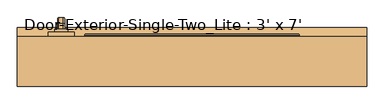
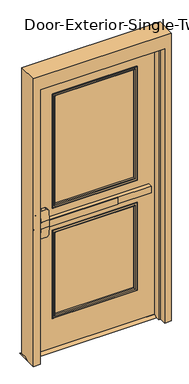
"""IFC4 building model written with IfcOpenShell, lengths in millimetres: door geometry, Door-Exterior-Single-Two_Lite : 3' x 7'."""

from ifc_helpers import new_model, si_unit, point, frame, frame_2d, origin, place, context, project, spatial, polyline, circle_curve, ellipse_curve, trimmed, segment, composite_curve, outline, extrude, faceted_brep, source, transform, mapped, element, save
from ifc_brep_helpers import plane_surface, cylinder_surface, revolved_surface, advanced_brep


def door_exterior_single_two_lite_3_x_7_37050820(model_context):
    return source(origin(), model_context, "Body", "SolidModel", [
        extrude(outline(polyline([(12.7, 12.7), (57.15, 12.7), (82.55, 0.0), (-12.7, 0.0), (12.7, 12.7)])), frame((-508.0, 0.0, 0.0), z_axis=(1.0, 0.0, 0.0), x_axis=(0.0, 1.0, 0.0)), (0.0, 0.0, 1.0), 1016.0),
        extrude(outline(polyline([(150.2833333, -25.4), (-349.25, -25.4), (-349.25, -19.05), (150.2833333, -19.05), (150.2833333, -25.4)])), frame((0.0, 0.0, 990.6), z_axis=(0.0, 0.0, 1.0), x_axis=(1.0, 0.0, 0.0)), (0.0, 0.0, 1.0), 50.8),
        advanced_brep(
        [(-412.75, -19.05, 1041.4), (-412.75, -19.05, 990.6), (-349.25, -19.05, 990.6), (400.05, -19.05, 990.6), (400.05, -19.05, 1041.4), (-349.25, -19.05, 1041.4), (400.05, 12.7, 1041.4), (400.05, 12.7, 990.6), (-349.25, 12.7, 990.6), (-349.25, 12.7, 927.1), (-368.3, 12.7, 908.05), (-393.7, 12.7, 908.05), (-412.75, 12.7, 927.1), (-412.75, 12.7, 1104.9), (-393.7, 12.7, 1123.95), (-368.3, 12.7, 1123.95), (-349.25, 12.7, 1104.9), (-349.25, 12.7, 1041.4), (-349.25, -15.8747533, 1041.4), (-412.75, -15.8747533, 1041.4), (-412.75, -10.8645731, 1104.9), (-412.75, -10.8645731, 927.1), (-412.75, -15.8747533, 990.6), (-349.25, -15.8747533, 990.6), (-349.25, -10.8645731, 927.1), (-349.25, -10.8645731, 1104.9), (-393.7, -9.361519, 1123.95), (-368.3, -9.361519, 1123.95), (-368.3, -9.361519, 908.05), (-393.7, -9.361519, 908.05)],
        [
            (0, 1),
            (1, 2),
            (2, 3),
            (3, 4),
            (4, 5),
            (5, 0),
            (6, 7),
            (7, 8),
            (8, 9),
            (9, 10, circle_curve(frame((-368.3, 12.7, 927.1), z_axis=(0.0, 1.0, 0.0), x_axis=(1.0, 0.0, 0.0)), 19.05)),
            (10, 11),
            (11, 12, circle_curve(frame((-393.7, 12.7, 927.1), z_axis=(0.0, 1.0, 0.0), x_axis=(1.0, 0.0, 0.0)), 19.05)),
            (12, 13),
            (13, 14, circle_curve(frame((-393.7, 12.7, 1104.9), z_axis=(0.0, 1.0, 0.0), x_axis=(1.0, 0.0, 0.0)), 19.05)),
            (14, 15),
            (15, 16, circle_curve(frame((-368.3, 12.7, 1104.9), z_axis=(0.0, 1.0, 0.0), x_axis=(1.0, 0.0, 0.0)), 19.05)),
            (16, 17),
            (17, 6),
            (4, 6),
            (17, 18),
            (18, 19),
            (19, 0),
            (19, 20),
            (20, 13),
            (12, 21),
            (21, 22),
            (22, 1),
            (7, 3),
            (22, 23),
            (23, 8),
            (23, 24),
            (24, 9),
            (16, 25),
            (25, 18),
            (14, 26),
            (26, 27),
            (27, 15),
            (10, 28),
            (28, 29),
            (29, 11),
            (24, 28, ellipse_curve(frame((-368.3, -10.8645731, 927.1), z_axis=(0.0, 0.9969018152893365, 0.07865602756830282), x_axis=(0.0, -0.07865602756830208, 0.9969018152893365)), 19.1092038, 19.05)),
            (27, 25, ellipse_curve(frame((-368.3, -10.8645731, 1104.9), z_axis=(0.0, 0.9969018152893376, -0.07865602756828934), x_axis=(0.0, -0.078656027568288, -0.9969018152893377)), 19.1092038, 19.05)),
            (20, 26, ellipse_curve(frame((-393.7, -10.8645731, 1104.9), z_axis=(0.0, 0.9969018152893376, -0.07865602756828934), x_axis=(0.0, -0.078656027568288, -0.9969018152893377)), 19.1092038, 19.05)),
            (29, 21, ellipse_curve(frame((-393.7, -10.8645731, 927.1), z_axis=(0.0, 0.9969018152893365, 0.07865602756830282), x_axis=(0.0, -0.07865602756830208, 0.9969018152893365)), 19.1092038, 19.05)),
        ],
        [
            plane_surface(frame((-412.75, -19.05, 1041.4), z_axis=(0.0, -1.0, 0.0), x_axis=(-1.0, 0.0, 0.0))),
            plane_surface(frame((-412.75, 12.7, 1041.4), z_axis=(0.0, 1.0, 0.0), x_axis=(1.0, 0.0, 0.0))),
            plane_surface(frame((400.05, -19.05, 1041.4), z_axis=(0.0, 0.0, 1.0), x_axis=(0.0, 1.0, 0.0))),
            plane_surface(frame((-412.75, -19.05, 1041.4), z_axis=(-1.0, 0.0, 0.0), x_axis=(0.0, 1.0, 0.0))),
            plane_surface(frame((-412.75, -19.05, 990.6), z_axis=(0.0, 0.0, -1.0), x_axis=(0.0, 1.0, 0.0))),
            plane_surface(frame((400.05, -19.05, 990.6), z_axis=(1.0, 0.0, 0.0), x_axis=(0.0, 1.0, 0.0))),
            plane_surface(frame((-349.25, -15.8747533, 927.1), z_axis=(1.0, 0.0, 0.0), x_axis=(0.0, 1.0, 0.0))),
            plane_surface(frame((-368.3, -15.8747533, 1123.95), z_axis=(0.0, 0.0, 1.0), x_axis=(0.0, 1.0, 0.0))),
            plane_surface(frame((-393.7, -15.8747533, 908.05), z_axis=(0.0, 0.0, -1.0), x_axis=(0.0, 1.0, 0.0))),
            cylinder_surface(frame((-368.3, 12.7, 927.1), z_axis=(0.0, -1.0, 0.0), x_axis=(1.0, 0.0, 0.0)), 19.05),
            cylinder_surface(frame((-368.3, 12.7, 1104.9), z_axis=(0.0, -1.0, 0.0), x_axis=(1.0, 0.0, 0.0)), 19.05),
            cylinder_surface(frame((-393.7, 12.7, 1104.9), z_axis=(0.0, -1.0, 0.0), x_axis=(1.0, 0.0, 0.0)), 19.05),
            cylinder_surface(frame((-393.7, 12.7, 927.1), z_axis=(0.0, -1.0, 0.0), x_axis=(1.0, 0.0, 0.0)), 19.05),
            plane_surface(frame((-349.25, -15.8747533, 1041.4), z_axis=(0.0, -0.9969018152893376, 0.07865602756828934), x_axis=(-1.0, 0.0, 0.0))),
            plane_surface(frame((-349.25, -9.361519, 908.05), z_axis=(0.0, -0.9969018152893365, -0.07865602756830282), x_axis=(-1.0, 0.0, 0.0))),
        ],
        [
            (0, [[1, 2, 3, 4, 5, 6]]),
            (1, [[7, 8, 9, 10, 11, 12, 13, 14, 15, 16, 17, 18]]),
            (2, [[19, -18, 20, 21, 22, -6, -5]]),
            (3, [[-1, -22, 23, 24, -13, 25, 26, 27]]),
            (4, [[28, -3, -2, -27, 29, 30, -8]]),
            (5, [[-4, -28, -7, -19]]),
            (6, [[-9, -30, 31, 32]]),
            (6, [[-17, 33, 34, -20]]),
            (7, [[-15, 35, 36, 37]]),
            (8, [[-11, 38, 39, 40]]),
            (9, [[-10, -32, 41, -38]]),
            (10, [[-16, -37, 42, -33]]),
            (11, [[-14, -24, 43, -35]]),
            (12, [[-12, -40, 44, -25]]),
            (13, [[-21, -34, -42, -36, -43, -23]]),
            (14, [[-26, -44, -39, -41, -31, -29]]),
        ],
    ),
        advanced_brep(
        [(-391.0, 69.85, 1017.190625), (-391.0, 69.85, 1014.809375), (-387.428125, 69.85, 1011.2375), (-374.5715406, 69.85, 1011.2375), (-371.0, 69.85, 1014.8090406), (-371.0, 69.85, 1017.190625), (-374.571875, 69.85, 1020.7625), (-387.428125, 69.85, 1020.7625), (-391.0, 69.85, 887.809375), (-387.428125, 69.85, 884.2375), (-374.571875, 69.85, 884.2375), (-371.0, 69.85, 887.809375), (-371.0, 69.85, 890.1909594), (-374.5715406, 69.85, 893.7625), (-387.428125, 69.85, 893.7625), (-391.0, 69.85, 890.190625), (-391.0, 95.25, 1017.190625), (-391.0, 109.140625, 1003.3), (-391.0, 109.140625, 901.7), (-391.0, 95.25, 887.809375), (-391.0, 95.25, 890.190625), (-391.0, 106.759375, 901.7), (-391.0, 106.759375, 1003.3), (-391.0, 95.25, 1014.809375), (-387.428125, 95.25, 1011.2375), (-374.5715406, 95.25, 1011.2375), (-371.0, 95.25, 1014.8090406), (-371.0, 106.7590406, 1003.3), (-371.0, 106.7590406, 901.7), (-371.0, 95.25, 890.1909594), (-371.0, 95.25, 887.809375), (-371.0, 109.140625, 901.7), (-371.0, 109.140625, 1003.3), (-371.0, 95.25, 1017.190625), (-374.571875, 95.25, 1020.7625), (-387.428125, 95.25, 1020.7625), (-387.428125, 103.1875, 1003.3), (-374.5715406, 103.1875, 1003.3), (-374.571875, 112.7125, 1003.3), (-387.428125, 112.7125, 1003.3), (-387.428125, 103.1875, 901.7), (-374.5715406, 103.1875, 901.7), (-374.571875, 112.7125, 901.7), (-387.428125, 112.7125, 901.7), (-387.428125, 95.25, 893.7625), (-374.5715406, 95.25, 893.7625), (-374.571875, 95.25, 884.2375), (-387.428125, 95.25, 884.2375)],
        [
            (0, 1),
            (1, 2, circle_curve(frame((-387.428125, 69.85, 1014.809375), z_axis=(0.0, -1.0, 0.0), x_axis=(0.0, 0.0, 1.0)), 3.571875)),
            (2, 3),
            (3, 4, circle_curve(frame((-374.5715406, 69.85, 1014.8090406), z_axis=(0.0, -1.0, 0.0), x_axis=(0.0, 0.0, 1.0)), 3.5715406)),
            (4, 5),
            (5, 6, circle_curve(frame((-374.571875, 69.85, 1017.190625), z_axis=(0.0, -1.0, 0.0), x_axis=(0.0, 0.0, 1.0)), 3.571875)),
            (6, 7),
            (7, 0, circle_curve(frame((-387.428125, 69.85, 1017.190625), z_axis=(0.0, -1.0, 0.0), x_axis=(0.0, 0.0, 1.0)), 3.571875)),
            (8, 9, circle_curve(frame((-387.428125, 69.85, 887.809375), z_axis=(0.0, -1.0, 0.0), x_axis=(0.0, 0.0, -1.0)), 3.571875)),
            (9, 10),
            (10, 11, circle_curve(frame((-374.571875, 69.85, 887.809375), z_axis=(0.0, -1.0, 0.0), x_axis=(0.0, 0.0, -1.0)), 3.571875)),
            (11, 12),
            (12, 13, circle_curve(frame((-374.5715406, 69.85, 890.1909594), z_axis=(0.0, -1.0, 0.0), x_axis=(0.0, 0.0, -1.0)), 3.5715406)),
            (13, 14),
            (14, 15, circle_curve(frame((-387.428125, 69.85, 890.190625), z_axis=(0.0, -1.0, 0.0), x_axis=(0.0, 0.0, -1.0)), 3.571875)),
            (15, 8),
            (0, 16),
            (16, 17, circle_curve(frame((-391.0, 95.25, 1003.3), z_axis=(-1.0, 0.0, 0.0), x_axis=(0.0, 0.0, 1.0)), 13.890625)),
            (17, 18),
            (18, 19, circle_curve(frame((-391.0, 95.25, 901.7), z_axis=(-1.0, 0.0, 0.0), x_axis=(0.0, 1.0, 0.0)), 13.890625)),
            (19, 8),
            (15, 20),
            (20, 21, circle_curve(frame((-391.0, 95.25, 901.7), z_axis=(1.0, 0.0, 0.0), x_axis=(0.0, 1.0, 0.0)), 11.509375)),
            (21, 22),
            (22, 23, circle_curve(frame((-391.0, 95.25, 1003.3), z_axis=(1.0, 0.0, 0.0), x_axis=(0.0, 0.0, 1.0)), 11.509375)),
            (23, 1),
            (23, 24, circle_curve(frame((-387.428125, 95.25, 1014.809375), z_axis=(0.0, -1.0, 0.0), x_axis=(0.0, 0.0, 1.0)), 3.571875)),
            (24, 2),
            (24, 25),
            (25, 3),
            (25, 26, circle_curve(frame((-374.5715406, 95.25, 1014.8090406), z_axis=(0.0, -1.0, 0.0), x_axis=(0.0, 0.0, 1.0)), 3.5715406)),
            (26, 4),
            (26, 27, circle_curve(frame((-371.0, 95.25, 1003.3), z_axis=(-1.0, 0.0, 0.0), x_axis=(0.0, 0.0, 1.0)), 11.5090406)),
            (27, 28),
            (28, 29, circle_curve(frame((-371.0, 95.25, 901.7), z_axis=(-1.0, 0.0, 0.0), x_axis=(0.0, 1.0, 0.0)), 11.5090406)),
            (29, 12),
            (11, 30),
            (30, 31, circle_curve(frame((-371.0, 95.25, 901.7), z_axis=(1.0, 0.0, 0.0), x_axis=(0.0, 1.0, 0.0)), 13.890625)),
            (31, 32),
            (32, 33, circle_curve(frame((-371.0, 95.25, 1003.3), z_axis=(1.0, 0.0, 0.0), x_axis=(0.0, 0.0, 1.0)), 13.890625)),
            (33, 5),
            (33, 34, circle_curve(frame((-374.571875, 95.25, 1017.190625), z_axis=(0.0, -1.0, 0.0), x_axis=(0.0, 0.0, 1.0)), 3.571875)),
            (34, 6),
            (34, 35),
            (35, 7),
            (35, 16, circle_curve(frame((-387.428125, 95.25, 1017.190625), z_axis=(0.0, -1.0, 0.0), x_axis=(0.0, 0.0, 1.0)), 3.571875)),
            (36, 24, circle_curve(frame((-387.428125, 95.25, 1003.3), z_axis=(1.0, 0.0, 0.0), x_axis=(0.0, 0.0, 1.0)), 7.9375)),
            (22, 36, circle_curve(frame((-387.428125, 106.759375, 1003.3), z_axis=(0.0, 0.0, 1.0), x_axis=(0.0, 1.0, 0.0)), 3.571875)),
            (37, 25, circle_curve(frame((-374.5715406, 95.25, 1003.3), z_axis=(1.0, 0.0, 0.0), x_axis=(0.0, 0.0, 1.0)), 7.9375)),
            (36, 37),
            (37, 27, circle_curve(frame((-374.5715406, 106.7590406, 1003.3), z_axis=(0.0, 0.0, 1.0), x_axis=(0.0, 1.0, 0.0)), 3.5715406)),
            (38, 34, circle_curve(frame((-374.571875, 95.25, 1003.3), z_axis=(1.0, 0.0, 0.0), x_axis=(0.0, 0.0, 1.0)), 17.4625)),
            (32, 38, circle_curve(frame((-374.571875, 109.140625, 1003.3), z_axis=(0.0, 0.0, 1.0), x_axis=(0.0, 1.0, 0.0)), 3.571875)),
            (39, 35, circle_curve(frame((-387.428125, 95.25, 1003.3), z_axis=(1.0, 0.0, 0.0), x_axis=(0.0, 0.0, 1.0)), 17.4625)),
            (38, 39),
            (39, 17, circle_curve(frame((-387.428125, 109.140625, 1003.3), z_axis=(0.0, 0.0, 1.0), x_axis=(0.0, 1.0, 0.0)), 3.571875)),
            (21, 40, circle_curve(frame((-387.428125, 106.759375, 901.7), z_axis=(0.0, 0.0, 1.0), x_axis=(0.0, 1.0, 0.0)), 3.571875)),
            (40, 36),
            (40, 41),
            (41, 37),
            (41, 28, circle_curve(frame((-374.5715406, 106.7590406, 901.7), z_axis=(0.0, 0.0, 1.0), x_axis=(0.0, 1.0, 0.0)), 3.5715406)),
            (31, 42, circle_curve(frame((-374.571875, 109.140625, 901.7), z_axis=(0.0, 0.0, 1.0), x_axis=(0.0, 1.0, 0.0)), 3.571875)),
            (42, 38),
            (42, 43),
            (43, 39),
            (43, 18, circle_curve(frame((-387.428125, 109.140625, 901.7), z_axis=(0.0, 0.0, 1.0), x_axis=(0.0, 1.0, 0.0)), 3.571875)),
            (44, 40, circle_curve(frame((-387.428125, 95.25, 901.7), z_axis=(1.0, 0.0, 0.0), x_axis=(0.0, 1.0, 0.0)), 7.9375)),
            (20, 44, circle_curve(frame((-387.428125, 95.25, 890.190625), z_axis=(0.0, 1.0, 0.0), x_axis=(0.0, 0.0, -1.0)), 3.571875)),
            (45, 41, circle_curve(frame((-374.5715406, 95.25, 901.7), z_axis=(1.0, 0.0, 0.0), x_axis=(0.0, 1.0, 0.0)), 7.9375)),
            (44, 45),
            (45, 29, circle_curve(frame((-374.5715406, 95.25, 890.1909594), z_axis=(0.0, 1.0, 0.0), x_axis=(0.0, 0.0, -1.0)), 3.5715406)),
            (46, 42, circle_curve(frame((-374.571875, 95.25, 901.7), z_axis=(1.0, 0.0, 0.0), x_axis=(0.0, 1.0, 0.0)), 17.4625)),
            (30, 46, circle_curve(frame((-374.571875, 95.25, 887.809375), z_axis=(0.0, 1.0, 0.0), x_axis=(0.0, 0.0, -1.0)), 3.571875)),
            (47, 43, circle_curve(frame((-387.428125, 95.25, 901.7), z_axis=(1.0, 0.0, 0.0), x_axis=(0.0, 1.0, 0.0)), 17.4625)),
            (46, 47),
            (47, 19, circle_curve(frame((-387.428125, 95.25, 887.809375), z_axis=(0.0, 1.0, 0.0), x_axis=(0.0, 0.0, -1.0)), 3.571875)),
            (14, 44),
            (13, 45),
            (10, 46),
            (9, 47),
        ],
        [
            plane_surface(frame((-381.0, 69.85, 1016.0), z_axis=(0.0, -1.0, 0.0), x_axis=(1.0, 0.0, 0.0))),
            plane_surface(frame((-381.0, 69.85, 889.0), z_axis=(0.0, -1.0, 0.0), x_axis=(1.0, 0.0, 0.0))),
            plane_surface(frame((-391.0, 69.85, 1017.190625), z_axis=(-1.0, 0.0, 0.0), x_axis=(0.0, 1.0, 0.0))),
            cylinder_surface(frame((-387.428125, 69.85, 1014.809375), z_axis=(0.0, -1.0, 0.0), x_axis=(0.0, 0.0, 1.0)), 3.571875),
            plane_surface(frame((-387.428125, 69.85, 1011.2375), z_axis=(0.0, 0.0, -1.0), x_axis=(0.0, 1.0, 0.0))),
            cylinder_surface(frame((-374.5715406, 69.85, 1014.8090406), z_axis=(0.0, -1.0, 0.0), x_axis=(0.0, 0.0, 1.0)), 3.5715406),
            plane_surface(frame((-371.0, 69.85, 1014.8090406), z_axis=(1.0, 0.0, 0.0), x_axis=(0.0, 1.0, 0.0))),
            cylinder_surface(frame((-374.571875, 69.85, 1017.190625), z_axis=(0.0, -1.0, 0.0), x_axis=(0.0, 0.0, 1.0)), 3.571875),
            plane_surface(frame((-374.571875, 69.85, 1020.7625), z_axis=(0.0, 0.0, 1.0), x_axis=(0.0, 1.0, 0.0))),
            cylinder_surface(frame((-387.428125, 69.85, 1017.190625), z_axis=(0.0, -1.0, 0.0), x_axis=(0.0, 0.0, 1.0)), 3.571875),
            revolved_surface(trimmed(ellipse_curve(frame((-387.428125, 95.25, 1014.809375), z_axis=(0.0, -1.0, 0.0), x_axis=(0.0, 0.0, 1.0)), 3.571875, 3.571875), [point((-391.0, 95.25, 1014.809375))], [point((-387.428125, 95.25, 1011.2375))], True, "CARTESIAN"), (-381.0, 95.25, 1003.3), (-1.0, 0.0, 0.0)),
            revolved_surface(polyline([(-387.428125, 95.25, 1011.2375), (-374.5715406, 95.25, 1011.2375)]), (-381.0, 95.25, 1003.3), (-1.0, 0.0, 0.0)),
            revolved_surface(trimmed(ellipse_curve(frame((-374.5715406, 95.25, 1014.8090406), z_axis=(0.0, -1.0, 0.0), x_axis=(0.0, 0.0, 1.0)), 3.5715406, 3.5715406), [point((-374.5715406, 95.25, 1011.2375))], [point((-371.0, 95.25, 1014.8090406))], True, "CARTESIAN"), (-381.0, 95.25, 1003.3), (-1.0, 0.0, 0.0)),
            revolved_surface(trimmed(ellipse_curve(frame((-374.571875, 95.25, 1017.190625), z_axis=(0.0, -1.0, 0.0), x_axis=(0.0, 0.0, 1.0)), 3.571875, 3.571875), [point((-371.0, 95.25, 1017.190625))], [point((-374.571875, 95.25, 1020.7625))], True, "CARTESIAN"), (-381.0, 95.25, 1003.3), (-1.0, 0.0, 0.0)),
            cylinder_surface(frame((-381.0, 95.25, 1003.3), z_axis=(-1.0, 0.0, 0.0), x_axis=(0.0, 0.0, 1.0)), 17.4625),
            revolved_surface(trimmed(ellipse_curve(frame((-387.428125, 95.25, 1017.190625), z_axis=(0.0, -1.0, 0.0), x_axis=(0.0, 0.0, 1.0)), 3.571875, 3.571875), [point((-387.428125, 95.25, 1020.7625))], [point((-391.0, 95.25, 1017.190625))], True, "CARTESIAN"), (-381.0, 95.25, 1003.3), (-1.0, 0.0, 0.0)),
            cylinder_surface(frame((-387.428125, 106.759375, 1003.3), z_axis=(0.0, 0.0, 1.0), x_axis=(0.0, 1.0, 0.0)), 3.571875),
            plane_surface(frame((-387.428125, 103.1875, 1003.3), z_axis=(0.0, -1.0, 0.0), x_axis=(0.0, 0.0, -1.0))),
            cylinder_surface(frame((-374.5715406, 106.7590406, 1003.3), z_axis=(0.0, 0.0, 1.0), x_axis=(0.0, 1.0, 0.0)), 3.5715406),
            cylinder_surface(frame((-374.571875, 109.140625, 1003.3), z_axis=(0.0, 0.0, 1.0), x_axis=(0.0, 1.0, 0.0)), 3.571875),
            plane_surface(frame((-374.571875, 112.7125, 1003.3), z_axis=(0.0, 1.0, 0.0), x_axis=(0.0, 0.0, -1.0))),
            cylinder_surface(frame((-387.428125, 109.140625, 1003.3), z_axis=(0.0, 0.0, 1.0), x_axis=(0.0, 1.0, 0.0)), 3.571875),
            revolved_surface(trimmed(ellipse_curve(frame((-387.428125, 106.759375, 901.7), z_axis=(0.0, 0.0, 1.0), x_axis=(0.0, 1.0, 0.0)), 3.571875, 3.571875), [point((-391.0, 106.759375, 901.7))], [point((-387.428125, 103.1875, 901.7))], True, "CARTESIAN"), (-381.0, 95.25, 901.7), (-1.0, 0.0, 0.0)),
            revolved_surface(polyline([(-387.428125, 103.1875, 901.7), (-374.5715406, 103.1875, 901.7)]), (-381.0, 95.25, 901.7), (-1.0, 0.0, 0.0)),
            revolved_surface(trimmed(ellipse_curve(frame((-374.5715406, 106.7590406, 901.7), z_axis=(0.0, 0.0, 1.0), x_axis=(0.0, 1.0, 0.0)), 3.5715406, 3.5715406), [point((-374.5715406, 103.1875, 901.7))], [point((-371.0, 106.7590406, 901.7))], True, "CARTESIAN"), (-381.0, 95.25, 901.7), (-1.0, 0.0, 0.0)),
            revolved_surface(trimmed(ellipse_curve(frame((-374.571875, 109.140625, 901.7), z_axis=(0.0, 0.0, 1.0), x_axis=(0.0, 1.0, 0.0)), 3.571875, 3.571875), [point((-371.0, 109.140625, 901.7))], [point((-374.571875, 112.7125, 901.7))], True, "CARTESIAN"), (-381.0, 95.25, 901.7), (-1.0, 0.0, 0.0)),
            cylinder_surface(frame((-381.0, 95.25, 901.7), z_axis=(-1.0, 0.0, 0.0), x_axis=(0.0, 1.0, 0.0)), 17.4625),
            revolved_surface(trimmed(ellipse_curve(frame((-387.428125, 109.140625, 901.7), z_axis=(0.0, 0.0, 1.0), x_axis=(0.0, 1.0, 0.0)), 3.571875, 3.571875), [point((-387.428125, 112.7125, 901.7))], [point((-391.0, 109.140625, 901.7))], True, "CARTESIAN"), (-381.0, 95.25, 901.7), (-1.0, 0.0, 0.0)),
            cylinder_surface(frame((-387.428125, 95.25, 890.190625), z_axis=(0.0, 1.0, 0.0), x_axis=(0.0, 0.0, -1.0)), 3.571875),
            plane_surface(frame((-387.428125, 95.25, 893.7625), z_axis=(0.0, 0.0, 1.0), x_axis=(0.0, -1.0, 0.0))),
            cylinder_surface(frame((-374.5715406, 95.25, 890.1909594), z_axis=(0.0, 1.0, 0.0), x_axis=(0.0, 0.0, -1.0)), 3.5715406),
            cylinder_surface(frame((-374.571875, 95.25, 887.809375), z_axis=(0.0, 1.0, 0.0), x_axis=(0.0, 0.0, -1.0)), 3.571875),
            plane_surface(frame((-374.571875, 95.25, 884.2375), z_axis=(0.0, 0.0, -1.0), x_axis=(0.0, -1.0, 0.0))),
            cylinder_surface(frame((-387.428125, 95.25, 887.809375), z_axis=(0.0, 1.0, 0.0), x_axis=(0.0, 0.0, -1.0)), 3.571875),
        ],
        [
            (0, [[1, 2, 3, 4, 5, 6, 7, 8]]),
            (1, [[9, 10, 11, 12, 13, 14, 15, 16]]),
            (2, [[-1, 17, 18, 19, 20, 21, -16, 22, 23, 24, 25, 26]]),
            (3, [[-2, -26, 27, 28]]),
            (4, [[-3, -28, 29, 30]]),
            (5, [[-4, -30, 31, 32]]),
            (6, [[-5, -32, 33, 34, 35, 36, -12, 37, 38, 39, 40, 41]]),
            (7, [[-6, -41, 42, 43]]),
            (8, [[-7, -43, 44, 45]]),
            (9, [[-8, -45, 46, -17]]),
            (10, [[47, -27, -25, 48]]),
            (11, [[49, -29, -47, 50]]),
            (12, [[-33, -31, -49, 51]]),
            (13, [[52, -42, -40, 53]]),
            (14, [[54, -44, -52, 55]]),
            (15, [[-18, -46, -54, 56]]),
            (16, [[-48, -24, 57, 58]]),
            (17, [[-50, -58, 59, 60]]),
            (18, [[-51, -60, 61, -34]]),
            (19, [[-53, -39, 62, 63]]),
            (20, [[-55, -63, 64, 65]]),
            (21, [[-56, -65, 66, -19]]),
            (22, [[67, -57, -23, 68]]),
            (23, [[69, -59, -67, 70]]),
            (24, [[-35, -61, -69, 71]]),
            (25, [[72, -62, -38, 73]]),
            (26, [[74, -64, -72, 75]]),
            (27, [[-20, -66, -74, 76]]),
            (28, [[-68, -22, -15, 77]]),
            (29, [[-70, -77, -14, 78]]),
            (30, [[-71, -78, -13, -36]]),
            (31, [[-73, -37, -11, 79]]),
            (32, [[-75, -79, -10, 80]]),
            (33, [[-76, -80, -9, -21]]),
        ],
    ),
        extrude(outline(composite_curve([segment(trimmed(circle_curve(frame_2d((1117.6, -381.0)), 19.0), [point((1117.6, -400.0))], [point((1117.6, -362.0))], False, "CARTESIAN"), True, "CONTINUOUS"), segment(trimmed(circle_curve(frame_2d((1117.6, -381.0)), 19.0), [point((1117.6, -362.0))], [point((1117.6, -400.0))], False, "CARTESIAN"), True, "CONTINUOUS")], self_intersect=False)), frame((0.0, 69.85, 0.0), z_axis=(0.0, 1.0, 0.0), x_axis=(0.0, 0.0, 1.0)), (0.0, 0.0, 1.0), 8.73125),
        extrude(outline(composite_curve([segment(trimmed(circle_curve(frame_2d((1113.0338574, -381.0)), 89.3016225), [point((1193.8, -342.9))], [point((1193.8, -419.1))], False, "CARTESIAN"), True, "CONTINUOUS"), segment(polyline([(1193.8, -419.1), (838.2, -419.1)]), True, "CONTINUOUS"), segment(trimmed(circle_curve(frame_2d((918.9661426, -381.0)), 89.3016225), [point((838.2, -419.1))], [point((838.2, -342.9))], False, "CARTESIAN"), True, "CONTINUOUS"), segment(polyline([(838.2, -342.9), (1193.8, -342.9)]), True, "CONTINUOUS")], self_intersect=False)), frame((0.0, 57.15, 0.0), z_axis=(0.0, 1.0, 0.0), x_axis=(0.0, 0.0, 1.0)), (0.0, 0.0, 1.0), 12.7),
        extrude(outline(polyline([(2133.6, -457.2), (12.7, -457.2), (12.7, 457.2), (2133.6, 457.2), (2133.6, -457.2)]), holes=[polyline([(1981.2, -304.8), (1981.2, 304.8), (1111.25, 304.8), (1111.25, -304.8), (1981.2, -304.8)]), polyline([(920.75, -304.8), (920.75, 304.8), (254.0, 304.8), (254.0, -304.8), (920.75, -304.8)])]), frame((0.0, 12.7, 0.0), z_axis=(0.0, 1.0, 0.0), x_axis=(0.0, 0.0, 1.0)), (0.0, 0.0, 1.0), 44.45),
        faceted_brep([(457.2, 7.9375, 0.0), (457.2, 57.15, 0.0), (508.0, 57.15, 0.0), (508.0, -88.9, 0.0), (457.2, -88.9, 0.0), (457.2, -39.6875, 0.0), (441.325, -39.6875, 0.0), (441.325, 7.9375, 0.0), (457.2, 7.9375, 2133.6), (457.2, 57.15, 2133.6), (-457.2, 57.15, 2133.6), (-457.2, 57.15, 0.0), (-508.0, 57.15, 0.0), (-508.0, 57.15, 2235.2), (508.0, 57.15, 2235.2), (508.0, -88.9, 2235.2), (-508.0, -88.9, 2235.2), (-508.0, -88.9, 0.0), (-457.2, -88.9, 0.0), (-457.2, -88.9, 2133.6), (457.2, -88.9, 2133.6), (457.2, -39.6875, 2133.6), (-457.2, -39.6875, 2133.6), (-457.2, -39.6875, 0.0), (-441.325, -39.6875, 0.0), (-441.325, -39.6875, 2117.725), (441.325, -39.6875, 2117.725), (441.325, 7.9375, 2117.725), (-441.325, 7.9375, 2117.725), (-441.325, 7.9375, 0.0), (-457.2, 7.9375, 0.0), (-457.2, 7.9375, 2133.6)], [[[0, 1, 2, 3, 4, 5, 6, 7]], [[1, 0, 8, 9]], [[2, 1, 9, 10, 11, 12, 13, 14]], [[3, 2, 14, 15]], [[4, 3, 15, 16, 17, 18, 19, 20]], [[5, 4, 20, 21]], [[6, 5, 21, 22, 23, 24, 25, 26]], [[7, 6, 26, 27]], [[0, 7, 27, 28, 29, 30, 31, 8]], [[9, 8, 31, 10]], [[20, 19, 22, 21]], [[26, 25, 28, 27]], [[12, 11, 30, 29, 24, 23, 18, 17]], [[11, 10, 31, 30]], [[13, 12, 17, 16]], [[19, 18, 23, 22]], [[25, 24, 29, 28]], [[15, 14, 13, 16]]]),
        extrude(outline(polyline([(304.8, 25.4), (-304.8, 25.4), (-304.8, 44.45), (304.8, 44.45), (304.8, 25.4)])), frame((0.0, 0.0, 1111.25), z_axis=(0.0, 0.0, 1.0), x_axis=(1.0, 0.0, 0.0)), (0.0, 0.0, 1.0), 869.95),
        extrude(outline(polyline([(304.8, 25.4), (-304.8, 25.4), (-304.8, 44.45), (304.8, 44.45), (304.8, 25.4)])), frame((0.0, 0.0, 254.0), z_axis=(0.0, 0.0, 1.0), x_axis=(1.0, 0.0, 0.0)), (0.0, 0.0, 1.0), 666.75),
        advanced_brep(
        [(-304.8, 44.45, 1981.2), (-304.8, 57.15, 1981.2), (-304.8, 57.15, 1111.25), (-304.8, 44.45, 1111.25), (-292.8, 58.15, 1969.2), (-292.8, 44.45, 1969.2), (-292.8, 44.45, 1123.25), (-292.8, 58.15, 1123.25), (-297.8, 63.15, 1974.2), (-297.8, 63.15, 1118.25), (-312.8, 61.15, 1989.2), (-310.8, 63.15, 1987.2), (-310.8, 63.15, 1105.25), (-312.8, 61.15, 1103.25), (-312.8, 57.15, 1989.2), (-312.8, 57.15, 1103.25), (304.8, 57.15, 1111.25), (304.8, 44.45, 1111.25), (292.8, 44.45, 1123.25), (292.8, 58.15, 1123.25), (297.8, 63.15, 1118.25), (310.8, 63.15, 1105.25), (312.8, 61.15, 1103.25), (312.8, 57.15, 1103.25), (304.8, 57.15, 1981.2), (304.8, 44.45, 1981.2), (292.8, 44.45, 1969.2), (292.8, 58.15, 1969.2), (297.8, 63.15, 1974.2), (310.8, 63.15, 1987.2), (312.8, 61.15, 1989.2), (312.8, 57.15, 1989.2)],
        [
            (0, 1),
            (1, 2),
            (2, 3),
            (3, 0),
            (4, 5),
            (5, 6),
            (6, 7),
            (7, 4),
            (8, 4, ellipse_curve(frame((-297.8, 58.15, 1974.2), z_axis=(-0.7071067811865475, 0.0, -0.7071067811865475), x_axis=(-0.7071067811865474, 0.0, 0.7071067811865476)), 7.0710678, 5.0)),
            (7, 9, ellipse_curve(frame((-297.8, 58.15, 1118.25), z_axis=(-0.7071067811865475, 0.0, 0.7071067811865475), x_axis=(0.7071067811865474, 0.0, 0.7071067811865476)), 7.0710678, 5.0)),
            (9, 8),
            (10, 11, ellipse_curve(frame((-310.8, 61.15, 1987.2), z_axis=(-0.7071067811865475, 0.0, -0.7071067811865475), x_axis=(-0.7071067811865474, 0.0, 0.7071067811865476)), 2.8284271, 2.0)),
            (11, 12),
            (12, 13, ellipse_curve(frame((-310.8, 61.15, 1105.25), z_axis=(-0.7071067811865475, 0.0, 0.7071067811865475), x_axis=(0.7071067811865474, 0.0, 0.7071067811865476)), 2.8284271, 2.0)),
            (13, 10),
            (14, 10),
            (13, 15),
            (15, 14),
            (2, 16),
            (16, 17),
            (17, 3),
            (6, 18),
            (18, 19),
            (19, 7),
            (19, 20, ellipse_curve(frame((297.8, 58.15, 1118.25), z_axis=(-0.7071067811865475, 0.0, -0.7071067811865475), x_axis=(-0.7071067811865476, 0.0, 0.7071067811865474)), 7.0710678, 5.0)),
            (20, 9),
            (12, 21),
            (21, 22, ellipse_curve(frame((310.8, 61.15, 1105.25), z_axis=(-0.7071067811865475, 0.0, -0.7071067811865475), x_axis=(-0.7071067811865476, 0.0, 0.7071067811865474)), 2.8284271, 2.0)),
            (22, 13),
            (22, 23),
            (23, 15),
            (16, 24),
            (24, 25),
            (25, 17),
            (18, 26),
            (26, 27),
            (27, 19),
            (27, 28, ellipse_curve(frame((297.8, 58.15, 1974.2), z_axis=(0.7071067811865475, 0.0, -0.7071067811865475), x_axis=(-0.7071067811865474, 0.0, -0.7071067811865476)), 7.0710678, 5.0)),
            (28, 20),
            (21, 29),
            (29, 30, ellipse_curve(frame((310.8, 61.15, 1987.2), z_axis=(0.7071067811865475, 0.0, -0.7071067811865475), x_axis=(-0.7071067811865474, 0.0, -0.7071067811865476)), 2.8284271, 2.0)),
            (30, 22),
            (30, 31),
            (31, 23),
            (31, 14),
            (1, 24),
            (0, 25),
            (5, 26),
            (4, 27),
            (8, 28),
            (11, 29),
            (10, 30),
        ],
        [
            plane_surface(frame((-304.8, 57.15, 1981.2), z_axis=(-1.0, 0.0, 0.0), x_axis=(0.0, 0.0, -1.0))),
            plane_surface(frame((-292.8, 44.45, 1969.2), z_axis=(1.0, 0.0, 0.0), x_axis=(0.0, 0.0, -1.0))),
            cylinder_surface(frame((-297.8, 58.15, 1981.2), z_axis=(0.0, 0.0, 1.0), x_axis=(-1.0, 0.0, 0.0)), 5.0),
            cylinder_surface(frame((-310.8, 61.15, 1981.2), z_axis=(0.0, 0.0, 1.0), x_axis=(-1.0, 0.0, 0.0)), 2.0),
            plane_surface(frame((-312.8, 61.15, 1989.2), z_axis=(-1.0, 0.0, 0.0), x_axis=(0.0, 0.0, -1.0))),
            plane_surface(frame((-304.8, 57.15, 1111.25), z_axis=(0.0, 0.0, -1.0), x_axis=(1.0, 0.0, 0.0))),
            plane_surface(frame((-292.8, 44.45, 1123.25), z_axis=(0.0, 0.0, 1.0), x_axis=(1.0, 0.0, 0.0))),
            cylinder_surface(frame((-304.8, 58.15, 1118.25), z_axis=(-1.0, 0.0, 0.0), x_axis=(0.0, 0.0, -1.0)), 5.0),
            cylinder_surface(frame((-304.8, 61.15, 1105.25), z_axis=(-1.0, 0.0, 0.0), x_axis=(0.0, 0.0, -1.0)), 2.0),
            plane_surface(frame((-312.8, 61.15, 1103.25), z_axis=(0.0, 0.0, -1.0), x_axis=(1.0, 0.0, 0.0))),
            plane_surface(frame((304.8, 57.15, 1111.25), z_axis=(1.0, 0.0, 0.0), x_axis=(0.0, 0.0, 1.0))),
            plane_surface(frame((292.8, 44.45, 1123.25), z_axis=(-1.0, 0.0, 0.0), x_axis=(0.0, 0.0, 1.0))),
            cylinder_surface(frame((297.8, 58.15, 1111.25), z_axis=(0.0, 0.0, -1.0), x_axis=(1.0, 0.0, 0.0)), 5.0),
            cylinder_surface(frame((310.8, 61.15, 1111.25), z_axis=(0.0, 0.0, -1.0), x_axis=(1.0, 0.0, 0.0)), 2.0),
            plane_surface(frame((312.8, 61.15, 1103.25), z_axis=(1.0, 0.0, 0.0), x_axis=(0.0, 0.0, 1.0))),
            plane_surface(frame((312.8, 57.15, 1989.2), z_axis=(0.0, -1.0, 0.0), x_axis=(-1.0, 0.0, 0.0))),
            plane_surface(frame((304.8, 57.15, 1981.2), z_axis=(0.0, 0.0, 1.0), x_axis=(-1.0, 0.0, 0.0))),
            plane_surface(frame((304.8, 44.45, 1981.2), z_axis=(0.0, -1.0, 0.0), x_axis=(-1.0, 0.0, 0.0))),
            plane_surface(frame((292.8, 44.45, 1969.2), z_axis=(0.0, 0.0, -1.0), x_axis=(-1.0, 0.0, 0.0))),
            cylinder_surface(frame((304.8, 58.15, 1974.2), z_axis=(1.0, 0.0, 0.0), x_axis=(0.0, 0.0, 1.0)), 5.0),
            plane_surface(frame((297.8, 63.15, 1974.2), z_axis=(0.0, 1.0, 0.0), x_axis=(-1.0, 0.0, 0.0))),
            cylinder_surface(frame((304.8, 61.15, 1987.2), z_axis=(1.0, 0.0, 0.0), x_axis=(0.0, 0.0, 1.0)), 2.0),
            plane_surface(frame((312.8, 61.15, 1989.2), z_axis=(0.0, 0.0, 1.0), x_axis=(-1.0, 0.0, 0.0))),
        ],
        [
            (0, [[1, 2, 3, 4]]),
            (1, [[5, 6, 7, 8]]),
            (2, [[9, -8, 10, 11]]),
            (3, [[12, 13, 14, 15]]),
            (4, [[16, -15, 17, 18]]),
            (5, [[-3, 19, 20, 21]]),
            (6, [[-7, 22, 23, 24]]),
            (7, [[-10, -24, 25, 26]]),
            (8, [[-14, 27, 28, 29]]),
            (9, [[-17, -29, 30, 31]]),
            (10, [[-20, 32, 33, 34]]),
            (11, [[-23, 35, 36, 37]]),
            (12, [[-25, -37, 38, 39]]),
            (13, [[-28, 40, 41, 42]]),
            (14, [[-30, -42, 43, 44]]),
            (15, [[-31, -44, 45, -18], [46, -32, -19, -2]]),
            (16, [[-33, -46, -1, 47]]),
            (17, [[-21, -34, -47, -4], [48, -35, -22, -6]]),
            (18, [[-36, -48, -5, 49]]),
            (19, [[-38, -49, -9, 50]]),
            (20, [[51, -40, -27, -13], [-26, -39, -50, -11]]),
            (21, [[-41, -51, -12, 52]]),
            (22, [[-43, -52, -16, -45]]),
        ],
    ),
        advanced_brep(
        [(-304.8, 25.4, 1111.25), (-304.8, 12.7, 1111.25), (-304.8, 12.7, 1981.2), (-304.8, 25.4, 1981.2), (-292.8, 11.7, 1123.25), (-292.8, 25.4, 1123.25), (-292.8, 25.4, 1969.2), (-292.8, 11.7, 1969.2), (-297.8, 6.7, 1118.25), (-297.8, 6.7, 1974.2), (-312.8, 8.7, 1103.25), (-310.8, 6.7, 1105.25), (-310.8, 6.7, 1987.2), (-312.8, 8.7, 1989.2), (-312.8, 12.7, 1103.25), (-312.8, 12.7, 1989.2), (304.8, 12.7, 1981.2), (304.8, 25.4, 1981.2), (292.8, 25.4, 1969.2), (292.8, 11.7, 1969.2), (297.8, 6.7, 1974.2), (310.8, 6.7, 1987.2), (312.8, 8.7, 1989.2), (312.8, 12.7, 1989.2), (304.8, 12.7, 1111.25), (304.8, 25.4, 1111.25), (292.8, 25.4, 1123.25), (292.8, 11.7, 1123.25), (297.8, 6.7, 1118.25), (310.8, 6.7, 1105.25), (312.8, 8.7, 1103.25), (312.8, 12.7, 1103.25)],
        [
            (0, 1),
            (1, 2),
            (2, 3),
            (3, 0),
            (4, 5),
            (5, 6),
            (6, 7),
            (7, 4),
            (8, 4, ellipse_curve(frame((-297.8, 11.7, 1118.25), z_axis=(-0.7071067811865475, 0.0, 0.7071067811865475), x_axis=(-0.7071067811865474, 0.0, -0.7071067811865476)), 7.0710678, 5.0)),
            (7, 9, ellipse_curve(frame((-297.8, 11.7, 1974.2), z_axis=(-0.7071067811865475, 0.0, -0.7071067811865475), x_axis=(0.7071067811865474, 0.0, -0.7071067811865476)), 7.0710678, 5.0)),
            (9, 8),
            (10, 11, ellipse_curve(frame((-310.8, 8.7, 1105.25), z_axis=(-0.7071067811865475, 0.0, 0.7071067811865475), x_axis=(-0.7071067811865474, 0.0, -0.7071067811865476)), 2.8284271, 2.0)),
            (11, 12),
            (12, 13, ellipse_curve(frame((-310.8, 8.7, 1987.2), z_axis=(-0.7071067811865475, 0.0, -0.7071067811865475), x_axis=(0.7071067811865474, 0.0, -0.7071067811865476)), 2.8284271, 2.0)),
            (13, 10),
            (14, 10),
            (13, 15),
            (15, 14),
            (2, 16),
            (16, 17),
            (17, 3),
            (6, 18),
            (18, 19),
            (19, 7),
            (19, 20, ellipse_curve(frame((297.8, 11.7, 1974.2), z_axis=(-0.7071067811865475, 0.0, 0.7071067811865475), x_axis=(-0.7071067811865476, 0.0, -0.7071067811865474)), 7.0710678, 5.0)),
            (20, 9),
            (12, 21),
            (21, 22, ellipse_curve(frame((310.8, 8.7, 1987.2), z_axis=(-0.7071067811865475, 0.0, 0.7071067811865475), x_axis=(-0.7071067811865476, 0.0, -0.7071067811865474)), 2.8284271, 2.0)),
            (22, 13),
            (22, 23),
            (23, 15),
            (16, 24),
            (24, 25),
            (25, 17),
            (18, 26),
            (26, 27),
            (27, 19),
            (27, 28, ellipse_curve(frame((297.8, 11.7, 1118.25), z_axis=(0.7071067811865475, 0.0, 0.7071067811865475), x_axis=(-0.7071067811865474, 0.0, 0.7071067811865476)), 7.0710678, 5.0)),
            (28, 20),
            (21, 29),
            (29, 30, ellipse_curve(frame((310.8, 8.7, 1105.25), z_axis=(0.7071067811865475, 0.0, 0.7071067811865475), x_axis=(-0.7071067811865474, 0.0, 0.7071067811865476)), 2.8284271, 2.0)),
            (30, 22),
            (30, 31),
            (31, 23),
            (31, 14),
            (1, 24),
            (0, 25),
            (5, 26),
            (4, 27),
            (8, 28),
            (11, 29),
            (10, 30),
        ],
        [
            plane_surface(frame((-304.8, 12.7, 1111.25), z_axis=(-1.0, 0.0, 0.0), x_axis=(0.0, 0.0, 1.0))),
            plane_surface(frame((-292.8, 25.4, 1123.25), z_axis=(1.0, 0.0, 0.0), x_axis=(0.0, 0.0, 1.0))),
            cylinder_surface(frame((-297.8, 11.7, 1111.25), z_axis=(0.0, 0.0, -1.0), x_axis=(-1.0, 0.0, 0.0)), 5.0),
            cylinder_surface(frame((-310.8, 8.7, 1111.25), z_axis=(0.0, 0.0, -1.0), x_axis=(-1.0, 0.0, 0.0)), 2.0),
            plane_surface(frame((-312.8, 8.7, 1103.25), z_axis=(-1.0, 0.0, 0.0), x_axis=(0.0, 0.0, 1.0))),
            plane_surface(frame((-304.8, 12.7, 1981.2), z_axis=(0.0, 0.0, 1.0), x_axis=(1.0, 0.0, 0.0))),
            plane_surface(frame((-292.8, 25.4, 1969.2), z_axis=(0.0, 0.0, -1.0), x_axis=(1.0, 0.0, 0.0))),
            cylinder_surface(frame((-304.8, 11.7, 1974.2), z_axis=(-1.0, 0.0, 0.0), x_axis=(0.0, 0.0, 1.0)), 5.0),
            cylinder_surface(frame((-304.8, 8.7, 1987.2), z_axis=(-1.0, 0.0, 0.0), x_axis=(0.0, 0.0, 1.0)), 2.0),
            plane_surface(frame((-312.8, 8.7, 1989.2), z_axis=(0.0, 0.0, 1.0), x_axis=(1.0, 0.0, 0.0))),
            plane_surface(frame((304.8, 12.7, 1981.2), z_axis=(1.0, 0.0, 0.0), x_axis=(0.0, 0.0, -1.0))),
            plane_surface(frame((292.8, 25.4, 1969.2), z_axis=(-1.0, 0.0, 0.0), x_axis=(0.0, 0.0, -1.0))),
            cylinder_surface(frame((297.8, 11.7, 1981.2), z_axis=(0.0, 0.0, 1.0), x_axis=(1.0, 0.0, 0.0)), 5.0),
            cylinder_surface(frame((310.8, 8.7, 1981.2), z_axis=(0.0, 0.0, 1.0), x_axis=(1.0, 0.0, 0.0)), 2.0),
            plane_surface(frame((312.8, 8.7, 1989.2), z_axis=(1.0, 0.0, 0.0), x_axis=(0.0, 0.0, -1.0))),
            plane_surface(frame((312.8, 12.7, 1103.25), z_axis=(0.0, 1.0, 0.0), x_axis=(-1.0, 0.0, 0.0))),
            plane_surface(frame((304.8, 12.7, 1111.25), z_axis=(0.0, 0.0, -1.0), x_axis=(-1.0, 0.0, 0.0))),
            plane_surface(frame((304.8, 25.4, 1111.25), z_axis=(0.0, 1.0, 0.0), x_axis=(-1.0, 0.0, 0.0))),
            plane_surface(frame((292.8, 25.4, 1123.25), z_axis=(0.0, 0.0, 1.0), x_axis=(-1.0, 0.0, 0.0))),
            cylinder_surface(frame((304.8, 11.7, 1118.25), z_axis=(1.0, 0.0, 0.0), x_axis=(0.0, 0.0, -1.0)), 5.0),
            plane_surface(frame((297.8, 6.7, 1118.25), z_axis=(0.0, -1.0, 0.0), x_axis=(-1.0, 0.0, 0.0))),
            cylinder_surface(frame((304.8, 8.7, 1105.25), z_axis=(1.0, 0.0, 0.0), x_axis=(0.0, 0.0, -1.0)), 2.0),
            plane_surface(frame((312.8, 8.7, 1103.25), z_axis=(0.0, 0.0, -1.0), x_axis=(-1.0, 0.0, 0.0))),
        ],
        [
            (0, [[1, 2, 3, 4]]),
            (1, [[5, 6, 7, 8]]),
            (2, [[9, -8, 10, 11]]),
            (3, [[12, 13, 14, 15]]),
            (4, [[16, -15, 17, 18]]),
            (5, [[-3, 19, 20, 21]]),
            (6, [[-7, 22, 23, 24]]),
            (7, [[-10, -24, 25, 26]]),
            (8, [[-14, 27, 28, 29]]),
            (9, [[-17, -29, 30, 31]]),
            (10, [[-20, 32, 33, 34]]),
            (11, [[-23, 35, 36, 37]]),
            (12, [[-25, -37, 38, 39]]),
            (13, [[-28, 40, 41, 42]]),
            (14, [[-30, -42, 43, 44]]),
            (15, [[-31, -44, 45, -18], [46, -32, -19, -2]]),
            (16, [[-33, -46, -1, 47]]),
            (17, [[-21, -34, -47, -4], [48, -35, -22, -6]]),
            (18, [[-36, -48, -5, 49]]),
            (19, [[-38, -49, -9, 50]]),
            (20, [[51, -40, -27, -13], [-26, -39, -50, -11]]),
            (21, [[-41, -51, -12, 52]]),
            (22, [[-43, -52, -16, -45]]),
        ],
    ),
        advanced_brep(
        [(-304.8, 44.45, 920.75), (-304.8, 57.15, 920.75), (-304.8, 57.15, 254.0), (-304.8, 44.45, 254.0), (-292.8, 58.15, 908.75), (-292.8, 44.45, 908.75), (-292.8, 44.45, 266.0), (-292.8, 58.15, 266.0), (-297.8, 63.15, 913.75), (-297.8, 63.15, 261.0), (-312.8, 61.15, 928.75), (-310.8, 63.15, 926.75), (-310.8, 63.15, 248.0), (-312.8, 61.15, 246.0), (-312.8, 57.15, 928.75), (-312.8, 57.15, 246.0), (304.8, 57.15, 254.0), (304.8, 44.45, 254.0), (292.8, 44.45, 266.0), (292.8, 58.15, 266.0), (297.8, 63.15, 261.0), (310.8, 63.15, 248.0), (312.8, 61.15, 246.0), (312.8, 57.15, 246.0), (304.8, 57.15, 920.75), (304.8, 44.45, 920.75), (292.8, 44.45, 908.75), (292.8, 58.15, 908.75), (297.8, 63.15, 913.75), (310.8, 63.15, 926.75), (312.8, 61.15, 928.75), (312.8, 57.15, 928.75)],
        [
            (0, 1),
            (1, 2),
            (2, 3),
            (3, 0),
            (4, 5),
            (5, 6),
            (6, 7),
            (7, 4),
            (8, 4, ellipse_curve(frame((-297.8, 58.15, 913.75), z_axis=(-0.7071067811865475, 0.0, -0.7071067811865475), x_axis=(-0.7071067811865474, 0.0, 0.7071067811865476)), 7.0710678, 5.0)),
            (7, 9, ellipse_curve(frame((-297.8, 58.15, 261.0), z_axis=(-0.7071067811865475, 0.0, 0.7071067811865475), x_axis=(0.7071067811865474, 0.0, 0.7071067811865476)), 7.0710678, 5.0)),
            (9, 8),
            (10, 11, ellipse_curve(frame((-310.8, 61.15, 926.75), z_axis=(-0.7071067811865475, 0.0, -0.7071067811865475), x_axis=(-0.7071067811865474, 0.0, 0.7071067811865476)), 2.8284271, 2.0)),
            (11, 12),
            (12, 13, ellipse_curve(frame((-310.8, 61.15, 248.0), z_axis=(-0.7071067811865475, 0.0, 0.7071067811865475), x_axis=(0.7071067811865474, 0.0, 0.7071067811865476)), 2.8284271, 2.0)),
            (13, 10),
            (14, 10),
            (13, 15),
            (15, 14),
            (2, 16),
            (16, 17),
            (17, 3),
            (6, 18),
            (18, 19),
            (19, 7),
            (19, 20, ellipse_curve(frame((297.8, 58.15, 261.0), z_axis=(-0.7071067811865475, 0.0, -0.7071067811865475), x_axis=(-0.7071067811865476, 0.0, 0.7071067811865474)), 7.0710678, 5.0)),
            (20, 9),
            (12, 21),
            (21, 22, ellipse_curve(frame((310.8, 61.15, 248.0), z_axis=(-0.7071067811865475, 0.0, -0.7071067811865475), x_axis=(-0.7071067811865476, 0.0, 0.7071067811865474)), 2.8284271, 2.0)),
            (22, 13),
            (22, 23),
            (23, 15),
            (16, 24),
            (24, 25),
            (25, 17),
            (18, 26),
            (26, 27),
            (27, 19),
            (27, 28, ellipse_curve(frame((297.8, 58.15, 913.75), z_axis=(0.7071067811865475, 0.0, -0.7071067811865475), x_axis=(-0.7071067811865474, 0.0, -0.7071067811865476)), 7.0710678, 5.0)),
            (28, 20),
            (21, 29),
            (29, 30, ellipse_curve(frame((310.8, 61.15, 926.75), z_axis=(0.7071067811865475, 0.0, -0.7071067811865475), x_axis=(-0.7071067811865474, 0.0, -0.7071067811865476)), 2.8284271, 2.0)),
            (30, 22),
            (30, 31),
            (31, 23),
            (31, 14),
            (1, 24),
            (0, 25),
            (5, 26),
            (4, 27),
            (8, 28),
            (11, 29),
            (10, 30),
        ],
        [
            plane_surface(frame((-304.8, 57.15, 920.75), z_axis=(-1.0, 0.0, 0.0), x_axis=(0.0, 0.0, -1.0))),
            plane_surface(frame((-292.8, 44.45, 908.75), z_axis=(1.0, 0.0, 0.0), x_axis=(0.0, 0.0, -1.0))),
            cylinder_surface(frame((-297.8, 58.15, 920.75), z_axis=(0.0, 0.0, 1.0), x_axis=(-1.0, 0.0, 0.0)), 5.0),
            cylinder_surface(frame((-310.8, 61.15, 920.75), z_axis=(0.0, 0.0, 1.0), x_axis=(-1.0, 0.0, 0.0)), 2.0),
            plane_surface(frame((-312.8, 61.15, 928.75), z_axis=(-1.0, 0.0, 0.0), x_axis=(0.0, 0.0, -1.0))),
            plane_surface(frame((-304.8, 57.15, 254.0), z_axis=(0.0, 0.0, -1.0), x_axis=(1.0, 0.0, 0.0))),
            plane_surface(frame((-292.8, 44.45, 266.0), z_axis=(0.0, 0.0, 1.0), x_axis=(1.0, 0.0, 0.0))),
            cylinder_surface(frame((-304.8, 58.15, 261.0), z_axis=(-1.0, 0.0, 0.0), x_axis=(0.0, 0.0, -1.0)), 5.0),
            cylinder_surface(frame((-304.8, 61.15, 248.0), z_axis=(-1.0, 0.0, 0.0), x_axis=(0.0, 0.0, -1.0)), 2.0),
            plane_surface(frame((-312.8, 61.15, 246.0), z_axis=(0.0, 0.0, -1.0), x_axis=(1.0, 0.0, 0.0))),
            plane_surface(frame((304.8, 57.15, 254.0), z_axis=(1.0, 0.0, 0.0), x_axis=(0.0, 0.0, 1.0))),
            plane_surface(frame((292.8, 44.45, 266.0), z_axis=(-1.0, 0.0, 0.0), x_axis=(0.0, 0.0, 1.0))),
            cylinder_surface(frame((297.8, 58.15, 254.0), z_axis=(0.0, 0.0, -1.0), x_axis=(1.0, 0.0, 0.0)), 5.0),
            cylinder_surface(frame((310.8, 61.15, 254.0), z_axis=(0.0, 0.0, -1.0), x_axis=(1.0, 0.0, 0.0)), 2.0),
            plane_surface(frame((312.8, 61.15, 246.0), z_axis=(1.0, 0.0, 0.0), x_axis=(0.0, 0.0, 1.0))),
            plane_surface(frame((312.8, 57.15, 928.75), z_axis=(0.0, -1.0, 0.0), x_axis=(-1.0, 0.0, 0.0))),
            plane_surface(frame((304.8, 57.15, 920.75), z_axis=(0.0, 0.0, 1.0), x_axis=(-1.0, 0.0, 0.0))),
            plane_surface(frame((304.8, 44.45, 920.75), z_axis=(0.0, -1.0, 0.0), x_axis=(-1.0, 0.0, 0.0))),
            plane_surface(frame((292.8, 44.45, 908.75), z_axis=(0.0, 0.0, -1.0), x_axis=(-1.0, 0.0, 0.0))),
            cylinder_surface(frame((304.8, 58.15, 913.75), z_axis=(1.0, 0.0, 0.0), x_axis=(0.0, 0.0, 1.0)), 5.0),
            plane_surface(frame((297.8, 63.15, 913.75), z_axis=(0.0, 1.0, 0.0), x_axis=(-1.0, 0.0, 0.0))),
            cylinder_surface(frame((304.8, 61.15, 926.75), z_axis=(1.0, 0.0, 0.0), x_axis=(0.0, 0.0, 1.0)), 2.0),
            plane_surface(frame((312.8, 61.15, 928.75), z_axis=(0.0, 0.0, 1.0), x_axis=(-1.0, 0.0, 0.0))),
        ],
        [
            (0, [[1, 2, 3, 4]]),
            (1, [[5, 6, 7, 8]]),
            (2, [[9, -8, 10, 11]]),
            (3, [[12, 13, 14, 15]]),
            (4, [[16, -15, 17, 18]]),
            (5, [[-3, 19, 20, 21]]),
            (6, [[-7, 22, 23, 24]]),
            (7, [[-10, -24, 25, 26]]),
            (8, [[-14, 27, 28, 29]]),
            (9, [[-17, -29, 30, 31]]),
            (10, [[-20, 32, 33, 34]]),
            (11, [[-23, 35, 36, 37]]),
            (12, [[-25, -37, 38, 39]]),
            (13, [[-28, 40, 41, 42]]),
            (14, [[-30, -42, 43, 44]]),
            (15, [[-31, -44, 45, -18], [46, -32, -19, -2]]),
            (16, [[-33, -46, -1, 47]]),
            (17, [[-21, -34, -47, -4], [48, -35, -22, -6]]),
            (18, [[-36, -48, -5, 49]]),
            (19, [[-38, -49, -9, 50]]),
            (20, [[51, -40, -27, -13], [-26, -39, -50, -11]]),
            (21, [[-41, -51, -12, 52]]),
            (22, [[-43, -52, -16, -45]]),
        ],
    ),
        advanced_brep(
        [(304.8, 25.4, 920.75), (304.8, 12.7, 920.75), (304.8, 12.7, 254.0), (304.8, 25.4, 254.0), (292.8, 11.7, 908.75), (292.8, 25.4, 908.75), (292.8, 25.4, 266.0), (292.8, 11.7, 266.0), (297.8, 6.7, 913.75), (297.8, 6.7, 261.0), (312.8, 8.7, 928.75), (310.8, 6.7, 926.75), (310.8, 6.7, 248.0), (312.8, 8.7, 246.0), (312.8, 12.7, 928.75), (312.8, 12.7, 246.0), (-304.8, 12.7, 254.0), (-304.8, 25.4, 254.0), (-292.8, 25.4, 266.0), (-292.8, 11.7, 266.0), (-297.8, 6.7, 261.0), (-310.8, 6.7, 248.0), (-312.8, 8.7, 246.0), (-312.8, 12.7, 246.0), (-304.8, 12.7, 920.75), (-304.8, 25.4, 920.75), (-292.8, 25.4, 908.75), (-292.8, 11.7, 908.75), (-297.8, 6.7, 913.75), (-310.8, 6.7, 926.75), (-312.8, 8.7, 928.75), (-312.8, 12.7, 928.75)],
        [
            (0, 1),
            (1, 2),
            (2, 3),
            (3, 0),
            (4, 5),
            (5, 6),
            (6, 7),
            (7, 4),
            (8, 4, ellipse_curve(frame((297.8, 11.7, 913.75), z_axis=(0.7071067811865475, 0.0, -0.7071067811865475), x_axis=(0.7071067811865474, 0.0, 0.7071067811865476)), 7.0710678, 5.0)),
            (7, 9, ellipse_curve(frame((297.8, 11.7, 261.0), z_axis=(0.7071067811865475, 0.0, 0.7071067811865475), x_axis=(-0.7071067811865474, 0.0, 0.7071067811865476)), 7.0710678, 5.0)),
            (9, 8),
            (10, 11, ellipse_curve(frame((310.8, 8.7, 926.75), z_axis=(0.7071067811865475, 0.0, -0.7071067811865475), x_axis=(0.7071067811865474, 0.0, 0.7071067811865476)), 2.8284271, 2.0)),
            (11, 12),
            (12, 13, ellipse_curve(frame((310.8, 8.7, 248.0), z_axis=(0.7071067811865475, 0.0, 0.7071067811865475), x_axis=(-0.7071067811865474, 0.0, 0.7071067811865476)), 2.8284271, 2.0)),
            (13, 10),
            (14, 10),
            (13, 15),
            (15, 14),
            (2, 16),
            (16, 17),
            (17, 3),
            (6, 18),
            (18, 19),
            (19, 7),
            (19, 20, ellipse_curve(frame((-297.8, 11.7, 261.0), z_axis=(0.7071067811865475, 0.0, -0.7071067811865475), x_axis=(0.7071067811865476, 0.0, 0.7071067811865474)), 7.0710678, 5.0)),
            (20, 9),
            (12, 21),
            (21, 22, ellipse_curve(frame((-310.8, 8.7, 248.0), z_axis=(0.7071067811865475, 0.0, -0.7071067811865475), x_axis=(0.7071067811865476, 0.0, 0.7071067811865474)), 2.8284271, 2.0)),
            (22, 13),
            (22, 23),
            (23, 15),
            (16, 24),
            (24, 25),
            (25, 17),
            (18, 26),
            (26, 27),
            (27, 19),
            (27, 28, ellipse_curve(frame((-297.8, 11.7, 913.75), z_axis=(-0.7071067811865475, 0.0, -0.7071067811865475), x_axis=(0.7071067811865474, 0.0, -0.7071067811865476)), 7.0710678, 5.0)),
            (28, 20),
            (21, 29),
            (29, 30, ellipse_curve(frame((-310.8, 8.7, 926.75), z_axis=(-0.7071067811865475, 0.0, -0.7071067811865475), x_axis=(0.7071067811865474, 0.0, -0.7071067811865476)), 2.8284271, 2.0)),
            (30, 22),
            (30, 31),
            (31, 23),
            (31, 14),
            (1, 24),
            (0, 25),
            (5, 26),
            (4, 27),
            (8, 28),
            (11, 29),
            (10, 30),
        ],
        [
            plane_surface(frame((304.8, 12.7, 920.75), z_axis=(1.0, 0.0, 0.0), x_axis=(0.0, 0.0, -1.0))),
            plane_surface(frame((292.8, 25.4, 908.75), z_axis=(-1.0, 0.0, 0.0), x_axis=(0.0, 0.0, -1.0))),
            cylinder_surface(frame((297.8, 11.7, 920.75), z_axis=(0.0, 0.0, 1.0), x_axis=(1.0, 0.0, 0.0)), 5.0),
            cylinder_surface(frame((310.8, 8.7, 920.75), z_axis=(0.0, 0.0, 1.0), x_axis=(1.0, 0.0, 0.0)), 2.0),
            plane_surface(frame((312.8, 8.7, 928.75), z_axis=(1.0, 0.0, 0.0), x_axis=(0.0, 0.0, -1.0))),
            plane_surface(frame((304.8, 12.7, 254.0), z_axis=(0.0, 0.0, -1.0), x_axis=(-1.0, 0.0, 0.0))),
            plane_surface(frame((292.8, 25.4, 266.0), z_axis=(0.0, 0.0, 1.0), x_axis=(-1.0, 0.0, 0.0))),
            cylinder_surface(frame((304.8, 11.7, 261.0), z_axis=(1.0, 0.0, 0.0), x_axis=(0.0, 0.0, -1.0)), 5.0),
            cylinder_surface(frame((304.8, 8.7, 248.0), z_axis=(1.0, 0.0, 0.0), x_axis=(0.0, 0.0, -1.0)), 2.0),
            plane_surface(frame((312.8, 8.7, 246.0), z_axis=(0.0, 0.0, -1.0), x_axis=(-1.0, 0.0, 0.0))),
            plane_surface(frame((-304.8, 12.7, 254.0), z_axis=(-1.0, 0.0, 0.0), x_axis=(0.0, 0.0, 1.0))),
            plane_surface(frame((-292.8, 25.4, 266.0), z_axis=(1.0, 0.0, 0.0), x_axis=(0.0, 0.0, 1.0))),
            cylinder_surface(frame((-297.8, 11.7, 254.0), z_axis=(0.0, 0.0, -1.0), x_axis=(-1.0, 0.0, 0.0)), 5.0),
            cylinder_surface(frame((-310.8, 8.7, 254.0), z_axis=(0.0, 0.0, -1.0), x_axis=(-1.0, 0.0, 0.0)), 2.0),
            plane_surface(frame((-312.8, 8.7, 246.0), z_axis=(-1.0, 0.0, 0.0), x_axis=(0.0, 0.0, 1.0))),
            plane_surface(frame((-312.8, 12.7, 928.75), z_axis=(0.0, 1.0, 0.0), x_axis=(1.0, 0.0, 0.0))),
            plane_surface(frame((-304.8, 12.7, 920.75), z_axis=(0.0, 0.0, 1.0), x_axis=(1.0, 0.0, 0.0))),
            plane_surface(frame((-304.8, 25.4, 920.75), z_axis=(0.0, 1.0, 0.0), x_axis=(1.0, 0.0, 0.0))),
            plane_surface(frame((-292.8, 25.4, 908.75), z_axis=(0.0, 0.0, -1.0), x_axis=(1.0, 0.0, 0.0))),
            cylinder_surface(frame((-304.8, 11.7, 913.75), z_axis=(-1.0, 0.0, 0.0), x_axis=(0.0, 0.0, 1.0)), 5.0),
            plane_surface(frame((-297.8, 6.7, 913.75), z_axis=(0.0, -1.0, 0.0), x_axis=(1.0, 0.0, 0.0))),
            cylinder_surface(frame((-304.8, 8.7, 926.75), z_axis=(-1.0, 0.0, 0.0), x_axis=(0.0, 0.0, 1.0)), 2.0),
            plane_surface(frame((-312.8, 8.7, 928.75), z_axis=(0.0, 0.0, 1.0), x_axis=(1.0, 0.0, 0.0))),
        ],
        [
            (0, [[1, 2, 3, 4]]),
            (1, [[5, 6, 7, 8]]),
            (2, [[9, -8, 10, 11]]),
            (3, [[12, 13, 14, 15]]),
            (4, [[16, -15, 17, 18]]),
            (5, [[-3, 19, 20, 21]]),
            (6, [[-7, 22, 23, 24]]),
            (7, [[-10, -24, 25, 26]]),
            (8, [[-14, 27, 28, 29]]),
            (9, [[-17, -29, 30, 31]]),
            (10, [[-20, 32, 33, 34]]),
            (11, [[-23, 35, 36, 37]]),
            (12, [[-25, -37, 38, 39]]),
            (13, [[-28, 40, 41, 42]]),
            (14, [[-30, -42, 43, 44]]),
            (15, [[-31, -44, 45, -18], [46, -32, -19, -2]]),
            (16, [[-33, -46, -1, 47]]),
            (17, [[-21, -34, -47, -4], [48, -35, -22, -6]]),
            (18, [[-36, -48, -5, 49]]),
            (19, [[-38, -49, -9, 50]]),
            (20, [[51, -40, -27, -13], [-26, -39, -50, -11]]),
            (21, [[-41, -51, -12, 52]]),
            (22, [[-43, -52, -16, -45]]),
        ],
    ),
    ])


if __name__ == "__main__":
    model = new_model("IFC4")
    model_context = context("Model", 3, world=origin())
    ifc_project = project(units=[si_unit("LENGTHUNIT", "METRE", prefix="MILLI")], contexts=[model_context])
    site = spatial("IfcSite", under=ifc_project)
    building = spatial("IfcBuilding", under=site)
    placement = place(None, origin())
    door_exterior_single_two_lite_3_x_7_shape = door_exterior_single_two_lite_3_x_7_37050820(model_context)
    element("IfcDoor", 1, ObjectType="Door-Exterior-Single-Two_Lite : 3' x 7'", at=placement, inside=building, context=model_context, shape_type="MappedRepresentation", body=[
        mapped(door_exterior_single_two_lite_3_x_7_shape, transform((0.0, 0.0, 0.0), x_axis=(1.0, 0.0, 0.0), y_axis=(0.0, 1.0, 0.0), z_axis=(0.0, 0.0, 1.0))),
    ])
    save(model, "model.ifc")

# Revit data of these elements
# Type "Door-Exterior-Single-Two_Lite : 3' x 7'"
#   Type Mark = "19"
#   Assembly Code = "B2030100"
#   Analytic Construction = "Metal frame, double glass door"
#   Top Rail = 0' - 6"
#   Threshold Offset [instance default] = 0' - 0 1/2"
#   Threshold Length [instance default] = 3' - 4"
#   Thickness = 0' - 1 3/4"
#   Thermal Resistance (R) = 1.3794 (h·ft²·°F)/BTU
#   Swing Angle [instance default] = 90.00°
#   Strike Height = 3' - 4"
#   Stiles = 0' - 6"
#   Rough Width [instance default] = 3' - 4"
#   Rough Height [instance default] = 7' - 4"
#   MFOpeningHeight [instance default] = 0' - 4"
#   MFOpeningWidth [instance default] = 0' - 4"
#   Lock Rail = 0' - 7 1/2"
#   Heat Transfer Coefficient (U) = 0.7250 BTU/(h·ft²·°F)
#   Glass Thickness = 0' - 0 3/4"
#   Inset Calculate [instance default] = 0' - 4"
#   Masonry Inset [instance default] = 0' - 1"
#   Height = 7' - 0"
#   Width = 3' - 0"
#   Masonry Frame Depth = 0' - 5 3/4"
#   Bottom Rail = 0' - 10"
#   Masonry Frame [instance default] = yes
#   Function = 1
#   Threshold [instance default] = yes
#   Dry Wall Frame [instance default] = no
#   Threshold Material = none
#   Panic Bar Material = Metal - Stainless Steel
#   Panel Material = Metal - Painted - Grey
#   Glass Stop Material = Metal - Painted - Grey
#   Exterior Pull Material = Metal - Stainless Steel
#   Frame Material = Metal - Painted - Grey
#   Visual Light Transmittance = 0
#   Solar Heat Gain Coefficient = 0
#   Wall Closure = (empty or 0)
# Element 1 (IfcDoor, "Door-Exterior-Single-Two_Lite : 3' x 7'")
#   Materials on its faces: "Metal - Painted - Grey", "Metal - Stainless Steel", "Glass"
# Materials
#   "Metal - Stainless Steel": class "Metal", colour RGB 247 247 247, transparency 0
#   "Metal - Painted - Grey": class "Paint", colour RGB 104 104 104, transparency 0
#   "Glass": class "Glass", colour RGB 0 128 192, transparency 0.75, Description = "Soda Lime Glass", Cost = 0
